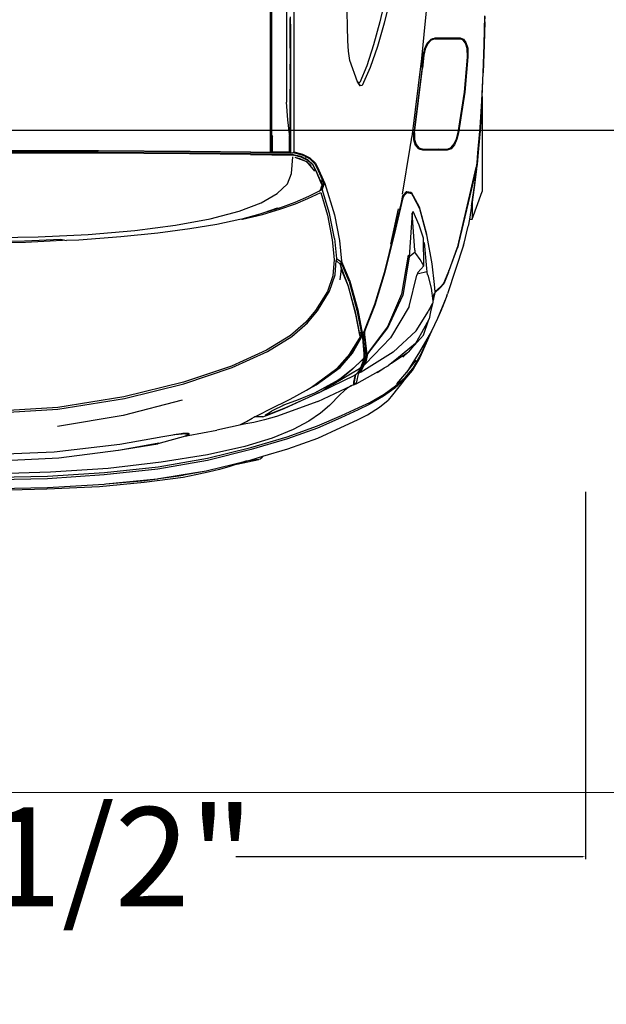
# Model space of a CAD drawing. Units: inches. Extents: x 1319 to 2030, y 219 to 1069.
# Tile 7 of 28: x 1464 to 1506, y 322 to 392. Entities that reach past the tile are written whole.
import ezdxf

# ---------------------------------------------------------------- set-up
doc = ezdxf.new("R2010")
doc.units = ezdxf.units.IN
doc.header["$MEASUREMENT"] = 0
doc.layers.get('0').update_dxf_attribs({"color": 12})
for name, color, linetype, lineweight in [('A-ANNO-DIMS', 2, 'Continuous', 18), ('A-FLOR', 8, 'Continuous', 18), ('C-PRKG-VEHC', 8, 'Continuous', 13)]:
    doc.layers.add(name, color=color, linetype=linetype, lineweight=lineweight)
doc.layers.add('Edges', color=250, linetype='Continuous')
doc.styles.get("Standard").update_dxf_attribs({"font": 'arial.ttf'})
doc.dimstyles.get("Standard").update_dxf_attribs({"dimtxt": 7, "dimasz": 0.18, "dimexe": 0.18, "dimexo": 0.0625, "dimgap": 0.09, "dimtad": 0, "dimtih": 1, "dimtoh": 1, "dimzin": 0, "dimdsep": 46, "dimlunit": 3, "dimtxsty": 'Standard', "dimcen": 0.09, "dimadec": 0, "dimazin": 0, "dimtfac": 1, "dimtofl": 0, "dimtmove": 0, "dimatfit": 3, "dimfxl": 1, "dimtolj": 1, "dimtzin": 0, "dimarcsym": 0})

# ---------------------------------------------------------------- blocks, each defined once
blk = doc.blocks.new('Nissan Qashqai pl')
at = {"layer": 'Edges'}
for p, q in [((10.8644, 12.8135), (10.8131, 12.8149)), ((10.8237, 12.8149), (10.8142, 12.8152)), ((10.8237, 12.8149), (10.864, 12.8138)), ((10.8596, 12.8138), (10.8589, 12.8138)), ((10.8642, 12.8136), (10.8596, 12.8138)), ((10.864, 12.8138), (10.8642, 12.8138)), ((10.8642, 12.8138), (10.9152, 12.812)), ((10.9158, 12.8118), (10.8644, 12.8135)), ((10.9577, 12.8101), (10.9152, 12.812)), ((10.9657, 12.8095), (10.9158, 12.8118)), ((10.9577, 12.8101), (10.9649, 12.8097)), ((10.9577, 12.8101), (11.1283, 12.8101)), ((10.9649, 12.8097), (11.0127, 12.8067)), ((11.0138, 12.8064), (10.9657, 12.8095)), ((11.0127, 12.8067), (11.0576, 12.8026)), ((11.059, 12.8023), (11.0138, 12.8064)), ((11.1783, 12.7921), (11.1283, 12.8101)), ((11.0576, 12.8026), (11.0798, 12.8008)), ((11.0768, 12.8008), (11.059, 12.8023)), ((11.0811, 12.8004), (11.0768, 12.8008)), ((11.0798, 12.8008), (11.0872, 12.7999)), ((11.0827, 12.8001), (11.0811, 12.8004)), ((11.0827, 12.8001), (11.0813, 12.7998)), ((11.0836, 12.8002), (11.0827, 12.8001)), ((11.0856, 12.7994), (11.0827, 12.8001)), ((11.0872, 12.7999), (11.0836, 12.8002)), ((11.0836, 12.8002), (11.0882, 12.7992)), ((11.2196, 12.7681), (11.0856, 12.7994)), ((11.0883, 12.7998), (11.0872, 12.7999)), ((11.0882, 12.7992), (11.2222, 12.7676)), ((11.0883, 12.7998), (11.1123, 12.797)), ((11.1147, 12.7965), (11.0883, 12.7998)), ((11.1123, 12.797), (11.1475, 12.7921)), ((11.1547, 12.791), (11.1147, 12.7965)), ((11.1475, 12.7921), (11.1525, 12.7914)), ((11.1475, 12.7921), (11.1783, 12.7921)), ((11.1525, 12.7914), (11.1547, 12.791)), ((11.1547, 12.791), (11.1783, 12.787)), ((11.1783, 12.787), (11.1783, 12.7921)), ((10.8523, 12.7704), (10.8546, 12.7762)), ((10.8523, 12.7255), (10.8523, 12.7704)), ((10.8543, 12.7702), (10.8538, 12.753)), ((10.8565, 12.7757), (10.8543, 12.7702)), ((10.8543, 12.7255), (10.8543, 12.7702)), ((10.8546, 12.7762), (10.8607, 12.7808)), ((10.8622, 12.7801), (10.8565, 12.7757)), ((10.8607, 12.7808), (10.8708, 12.7841)), ((10.8716, 12.7832), (10.8622, 12.7801)), ((10.8708, 12.7841), (10.8869, 12.7844)), ((10.887, 12.7835), (10.8716, 12.7832)), ((10.8869, 12.7844), (10.9499, 12.7789)), ((10.9498, 12.7781), (10.887, 12.7835)), ((11.0226, 12.7668), (10.9498, 12.7781)), ((10.9499, 12.7789), (11.0229, 12.7676)), ((11.1783, 12.787), (11.1906, 12.7849)), ((11.1906, 12.7849), (11.1909, 12.7849)), ((11.193, 12.7845), (11.1909, 12.7849)), ((11.2215, 12.7775), (11.193, 12.7845)), ((11.2247, 12.7764), (11.2215, 12.7775)), ((11.2247, 12.7764), (11.3124, 12.7479)), ((10.8528, 12.7503), (10.8535, 12.7521)), ((10.8535, 12.7521), (10.8538, 12.753)), ((10.8538, 12.7521), (10.8535, 12.7521)), ((10.8538, 12.753), (10.8538, 12.7521)), ((10.8538, 12.7521), (10.8538, 12.7502)), ((11.0339, 12.7639), (11.0226, 12.7668)), ((11.0229, 12.7676), (11.0348, 12.7645)), ((11.0429, 12.7597), (11.0339, 12.7639)), ((11.0348, 12.7645), (11.0444, 12.7601)), ((11.0497, 12.7542), (11.0429, 12.7597)), ((11.0444, 12.7601), (11.0516, 12.7542)), ((11.0523, 12.7475), (11.0497, 12.7542)), ((11.0516, 12.7542), (11.0543, 12.7473)), ((11.2247, 12.767), (11.2163, 12.7689)), ((11.22, 12.768), (11.2196, 12.7681)), ((11.2247, 12.767), (11.22, 12.768)), ((11.2222, 12.7676), (11.2271, 12.7664)), ((11.2253, 12.7668), (11.2247, 12.767)), ((11.2304, 12.7649), (11.2253, 12.7668)), ((11.2253, 12.7668), (11.2271, 12.7664)), ((11.2271, 12.7664), (11.2296, 12.7658)), ((11.2271, 12.7664), (11.2277, 12.7662)), ((11.2277, 12.7662), (11.2296, 12.7658)), ((11.2732, 12.7496), (11.2277, 12.7662)), ((11.2704, 12.7504), (11.2304, 12.7649)), ((10.8528, 12.742), (10.8528, 12.7503)), ((10.8528, 12.742), (10.8538, 12.742)), ((10.8528, 12.7419), (10.8528, 12.742)), ((10.8538, 12.7419), (10.8528, 12.7419)), ((10.8528, 12.7242), (10.8528, 12.7419)), ((10.8538, 12.7502), (10.8538, 12.742)), ((10.8538, 12.742), (10.8538, 12.7419)), ((10.8538, 12.7214), (10.8538, 12.7419)), ((11.0528, 12.73), (11.0523, 12.7475)), ((11.0523, 12.7312), (11.0523, 12.7475)), ((11.0543, 12.7473), (11.0543, 12.7035)), ((11.2702, 12.7507), (11.2704, 12.7504)), ((11.2704, 12.7506), (11.2707, 12.7503)), ((11.2707, 12.7503), (11.2704, 12.7504)), ((11.2719, 12.7498), (11.2707, 12.7503)), ((11.2934, 12.741), (11.2719, 12.7498)), ((11.2732, 12.7496), (11.2946, 12.7409)), ((11.3, 12.735), (11.2934, 12.741)), ((11.2946, 12.7409), (11.3018, 12.7346)), ((11.3081, 12.7253), (11.3, 12.735)), ((11.3018, 12.7346), (11.3103, 12.7249)), ((11.3161, 12.7467), (11.3124, 12.7479)), ((11.3161, 12.7467), (11.3376, 12.7381)), ((11.3192, 12.7454), (11.3566, 12.7294)), ((11.3405, 12.7369), (11.3376, 12.7381)), ((11.3405, 12.7369), (11.3566, 12.7294)), ((10.8528, 12.7242), (10.8523, 12.7255)), ((10.8538, 12.7214), (10.8528, 12.7242)), ((10.855, 12.7181), (10.8538, 12.7214)), ((10.8543, 12.7255), (10.8569, 12.7184)), ((10.8622, 12.7114), (10.855, 12.7181)), ((10.8569, 12.7184), (10.8637, 12.712)), ((11.0523, 12.7312), (11.0528, 12.73)), ((11.0523, 12.7287), (11.0523, 12.7312)), ((11.0528, 12.7274), (11.0523, 12.7287)), ((11.0523, 12.7037), (11.0523, 12.7287)), ((11.0528, 12.7274), (11.0528, 12.73)), ((11.0528, 12.73), (11.0538, 12.7273)), ((11.0528, 12.7274), (11.0528, 12.6985)), ((11.0538, 12.7273), (11.0538, 12.7018)), ((11.2091, 12.7103), (11.2583, 12.7196)), ((11.2583, 12.7196), (11.2956, 12.7234)), ((11.2787, 12.7123), (11.3022, 12.7186)), ((11.2956, 12.7234), (11.3085, 12.7247)), ((11.3022, 12.7186), (11.3252, 12.7213)), ((11.3086, 12.7247), (11.3081, 12.7253)), ((11.3081, 12.7253), (11.3087, 12.7247)), ((11.3085, 12.7247), (11.3086, 12.7247)), ((11.3086, 12.7247), (11.3087, 12.7247)), ((11.3087, 12.7247), (11.3103, 12.7249)), ((11.3103, 12.7249), (11.3103, 12.7249)), ((11.3103, 12.7249), (11.3106, 12.7249)), ((11.3106, 12.7249), (11.314, 12.7238)), ((11.317, 12.7227), (11.3119, 12.7236)), ((11.3132, 12.7243), (11.3256, 12.7215)), ((11.314, 12.7238), (11.317, 12.7227)), ((11.314, 12.7238), (11.3242, 12.7216)), ((11.3242, 12.7216), (11.317, 12.7227)), ((11.3198, 12.7211), (11.3252, 12.7213)), ((11.3242, 12.7216), (11.3256, 12.7215)), ((11.3252, 12.7213), (11.3283, 12.7214)), ((11.3256, 12.7215), (11.3283, 12.7214)), ((11.3283, 12.7214), (11.3297, 12.7206)), ((11.3297, 12.7206), (11.3446, 12.7173)), ((11.3297, 12.7206), (11.3302, 12.7203)), ((11.3302, 12.7203), (11.3446, 12.7173)), ((11.3302, 12.7203), (11.3394, 12.7152)), ((11.3446, 12.7173), (11.3571, 12.7146)), ((11.3566, 12.7294), (11.3796, 12.7187)), ((11.3796, 12.7187), (11.4164, 12.6974)), ((11.3796, 12.7187), (11.3807, 12.7182)), ((11.3807, 12.7182), (11.4267, 12.6979)), ((11.4228, 12.6989), (11.3807, 12.7182)), ((10.7615, 12.7131), (10.8218, 12.7077)), ((10.8218, 12.7077), (10.8896, 12.7008)), ((10.8718, 12.7068), (10.8622, 12.7114)), ((10.8637, 12.712), (10.8727, 12.7077)), ((10.8836, 12.7041), (10.8718, 12.7068)), ((10.8727, 12.7077), (10.8839, 12.7051)), ((10.9054, 12.702), (10.8836, 12.7041)), ((10.8839, 12.7051), (10.9067, 12.7029)), ((10.8896, 12.7008), (11.0304, 12.6838)), ((10.9054, 12.702), (11.0232, 12.6871)), ((11.0231, 12.6882), (10.9067, 12.7029)), ((11.0501, 12.6964), (11.0523, 12.7037)), ((11.0538, 12.7018), (11.0528, 12.6985)), ((11.0543, 12.7035), (11.0538, 12.7018)), ((11.156, 12.6966), (11.203, 12.7093)), ((11.1589, 12.6971), (11.2062, 12.7098)), ((11.2121, 12.7043), (11.189, 12.6968)), ((11.203, 12.7093), (11.2091, 12.7103)), ((11.2062, 12.7098), (11.2091, 12.7103)), ((11.2622, 12.7051), (11.2121, 12.7043)), ((11.2199, 12.706), (11.2666, 12.7097)), ((11.2601, 12.7037), (11.2505, 12.6987)), ((11.2622, 12.7051), (11.2601, 12.7037)), ((11.2743, 12.6942), (11.2622, 12.7051)), ((11.2666, 12.7097), (11.2729, 12.7104)), ((11.2787, 12.7123), (11.2729, 12.7104)), ((11.2729, 12.7104), (11.2766, 12.6957)), ((11.3394, 12.7152), (11.3434, 12.7138)), ((11.3394, 12.7152), (11.342, 12.7137)), ((11.379, 12.6915), (11.3434, 12.7138)), ((11.3583, 12.7142), (11.3571, 12.7146)), ((11.3571, 12.7146), (11.3821, 12.7008)), ((11.3583, 12.7142), (11.3821, 12.7008)), ((11.3864, 12.7044), (11.3583, 12.7142)), ((11.3821, 12.7008), (11.4014, 12.69)), ((11.4163, 12.6775), (11.3864, 12.7044)), ((11.0231, 12.6882), (11.035, 12.6883)), ((11.0358, 12.6872), (11.0232, 12.6871)), ((11.0357, 12.6829), (11.0304, 12.6838)), ((11.035, 12.6883), (11.0443, 12.6911)), ((11.0491, 12.6807), (11.0357, 12.6829)), ((11.0458, 12.6903), (11.0358, 12.6872)), ((11.0443, 12.6911), (11.0501, 12.6964)), ((11.052, 12.6958), (11.0458, 12.6903)), ((11.0528, 12.6985), (11.052, 12.6958)), ((11.1285, 12.6745), (11.1298, 12.6823)), ((11.1298, 12.6823), (11.156, 12.6966)), ((11.1306, 12.6752), (11.1319, 12.6827)), ((11.1319, 12.6827), (11.1306, 12.6812)), ((11.1319, 12.6827), (11.1365, 12.6851)), ((11.1365, 12.6851), (11.1589, 12.6971)), ((11.189, 12.6968), (11.1644, 12.6862)), ((11.1644, 12.6862), (11.1672, 12.6844)), ((11.2337, 12.6892), (11.1672, 12.6844)), ((11.1672, 12.6844), (11.2459, 12.6785)), ((11.2337, 12.6892), (11.2382, 12.6892)), ((11.2382, 12.6892), (11.2401, 12.6908)), ((11.2382, 12.6892), (11.2459, 12.6785)), ((11.2505, 12.6987), (11.2401, 12.6908)), ((11.2743, 12.6942), (11.2791, 12.6927)), ((11.335, 12.6786), (11.2791, 12.6927)), ((11.379, 12.6915), (11.417, 12.6499)), ((11.4014, 12.69), (11.4022, 12.6894)), ((11.4014, 12.69), (11.4265, 12.6594)), ((11.4022, 12.6894), (11.4163, 12.6775)), ((11.4022, 12.6894), (11.4265, 12.6594)), ((11.4164, 12.6974), (11.4531, 12.6744)), ((11.4243, 12.6982), (11.4228, 12.6989)), ((11.4464, 12.6853), (11.4243, 12.6982)), ((11.4267, 12.6979), (11.4498, 12.6844)), ((11.4531, 12.6744), (11.4314, 12.6911)), ((11.4624, 12.6717), (11.4464, 12.6853)), ((11.4498, 12.6844), (11.4662, 12.6706)), ((11.4681, 12.6691), (11.4498, 12.6844)), ((11.0449, 12.6812), (11.0448, 12.6812)), ((11.0492, 12.6807), (11.0491, 12.6807)), ((11.1336, 12.667), (11.0492, 12.6807)), ((11.1293, 12.6736), (11.1285, 12.6745)), ((11.1306, 12.6812), (11.1293, 12.6736)), ((11.1353, 12.6677), (11.1293, 12.6736)), ((11.1347, 12.671), (11.1306, 12.6752)), ((11.1366, 12.6691), (11.1347, 12.671)), ((11.1358, 12.6676), (11.1353, 12.6677)), ((11.1358, 12.6676), (11.1366, 12.6691)), ((11.148, 12.665), (11.1358, 12.6676)), ((11.1401, 12.6682), (11.1366, 12.6691)), ((11.2066, 12.6527), (11.1401, 12.6682)), ((11.2063, 12.6515), (11.148, 12.665)), ((11.2428, 12.6769), (11.3132, 12.6652)), ((11.2459, 12.6785), (11.3153, 12.6672)), ((11.3132, 12.6652), (11.3715, 12.6398)), ((11.3733, 12.6404), (11.3153, 12.6672)), ((11.335, 12.6786), (11.3915, 12.6453)), ((11.4366, 12.6471), (11.4163, 12.6775)), ((11.4163, 12.6775), (11.4259, 12.6674)), ((11.4742, 12.6567), (11.4531, 12.6744)), ((11.4774, 12.6543), (11.4624, 12.6717)), ((11.4662, 12.6706), (11.4815, 12.6531)), ((11.4681, 12.6691), (11.4936, 12.6491)), ((10.7776, 12.646), (10.8264, 12.6341)), ((11.2232, 12.6458), (11.1598, 12.6594)), ((11.272, 12.6349), (11.2063, 12.6515)), ((11.2728, 12.6357), (11.2066, 12.6527)), ((11.417, 12.6499), (11.4529, 12.5922)), ((11.4265, 12.6594), (11.4366, 12.6471)), ((11.4366, 12.6471), (11.4408, 12.6419)), ((11.4924, 12.6339), (11.4774, 12.6543)), ((11.4815, 12.6531), (11.4963, 12.6328)), ((11.4936, 12.6491), (11.5033, 12.6408)), ((10.7754, 12.637), (10.8239, 12.6261)), ((10.8264, 12.6341), (10.8682, 12.6216)), ((11.3311, 12.6172), (11.272, 12.6349)), ((11.3323, 12.6178), (11.2728, 12.6357)), ((11.3715, 12.6398), (11.4177, 12.6052)), ((11.4203, 12.6044), (11.3733, 12.6404)), ((11.3915, 12.6453), (11.4381, 12.6002)), ((11.4408, 12.6419), (11.4411, 12.6414)), ((11.4411, 12.6414), (11.4411, 12.6414)), ((11.4414, 12.6409), (11.4411, 12.6414)), ((11.4414, 12.6409), (11.447, 12.6315)), ((11.4455, 12.6336), (11.4414, 12.6409)), ((11.447, 12.6315), (11.4455, 12.6336)), ((11.4455, 12.6336), (11.4462, 12.6324)), ((11.447, 12.6315), (11.4462, 12.6324)), ((11.4732, 12.585), (11.4462, 12.6324)), ((11.447, 12.6315), (11.447, 12.6314)), ((11.4536, 12.6215), (11.447, 12.6314)), ((11.5074, 12.608), (11.4924, 12.6339)), ((11.4964, 12.6326), (11.4963, 12.6328)), ((11.4964, 12.6326), (11.5113, 12.6069)), ((11.5158, 12.6256), (11.5033, 12.6408)), ((10.8239, 12.6261), (10.8653, 12.6144)), ((10.8653, 12.6144), (10.9026, 12.6025)), ((10.8682, 12.6216), (10.9059, 12.6087)), ((11.3751, 12.5999), (11.3311, 12.6172)), ((11.3747, 12.6011), (11.3323, 12.6178)), ((11.5295, 12.6041), (11.5158, 12.6256)), ((10.9026, 12.6025), (10.933, 12.5901)), ((10.9059, 12.6087), (10.9384, 12.5945)), ((10.9384, 12.5945), (10.9386, 12.5905)), ((11.3411, 12.5863), (11.3795, 12.5939)), ((11.38, 12.5988), (11.3747, 12.6011)), ((11.3751, 12.5999), (11.3762, 12.5999)), ((11.3752, 12.5998), (11.3751, 12.5999)), ((11.3763, 12.5998), (11.3752, 12.5998)), ((11.3764, 12.5993), (11.3752, 12.5998)), ((11.3792, 12.5982), (11.3764, 12.5993)), ((11.3792, 12.5982), (11.3793, 12.5979)), ((11.3792, 12.5982), (11.3804, 12.5972)), ((11.3795, 12.5939), (11.3834, 12.5947)), ((11.3853, 12.5993), (11.38, 12.5988)), ((11.3804, 12.5972), (11.4082, 12.5998)), ((11.3827, 12.5953), (11.3804, 12.5972)), ((11.3804, 12.5926), (11.3841, 12.5933)), ((11.3811, 12.5958), (11.3808, 12.5961)), ((11.3834, 12.5947), (11.3827, 12.5953)), ((11.3846, 12.5953), (11.3829, 12.5952)), ((11.3829, 12.5952), (11.3849, 12.5951)), ((11.388, 12.591), (11.3829, 12.5952)), ((11.3834, 12.5947), (11.3841, 12.5933)), ((11.3846, 12.5953), (11.4248, 12.5976)), ((11.3846, 12.5953), (11.3846, 12.5953)), ((11.3851, 12.5951), (11.3846, 12.5953)), ((11.3846, 12.5953), (11.3849, 12.5951)), ((11.3849, 12.5951), (11.3851, 12.5951)), ((11.3882, 12.5923), (11.3849, 12.5951)), ((11.3851, 12.5951), (11.3867, 12.5949)), ((11.4171, 12.5766), (11.3851, 12.5951)), ((11.4212, 12.603), (11.3853, 12.5993)), ((11.3867, 12.5949), (11.3915, 12.5951)), ((11.3914, 12.5926), (11.3867, 12.5949)), ((11.3915, 12.5951), (11.4266, 12.5977)), ((11.409, 12.5999), (11.4082, 12.5998)), ((11.4164, 12.5998), (11.4082, 12.5998)), ((11.4152, 12.6004), (11.409, 12.5999)), ((11.409, 12.5999), (11.4163, 12.5999)), ((11.4173, 12.6006), (11.4152, 12.6004)), ((11.4163, 12.5999), (11.4152, 12.6004)), ((11.4163, 12.5999), (11.4186, 12.5999)), ((11.4164, 12.5998), (11.4163, 12.5999)), ((11.4181, 12.5998), (11.4164, 12.5998)), ((11.4169, 12.5996), (11.4164, 12.5998)), ((11.4252, 12.598), (11.4169, 12.5996)), ((11.4176, 12.6007), (11.4173, 12.6006)), ((11.418, 12.6006), (11.4173, 12.6006)), ((11.4215, 12.601), (11.4176, 12.6007)), ((11.418, 12.6006), (11.4176, 12.6007)), ((11.4177, 12.6052), (11.4193, 12.6042)), ((11.4204, 12.6002), (11.418, 12.6006)), ((11.4194, 12.6), (11.418, 12.6006)), ((11.4192, 12.6045), (11.4194, 12.6042)), ((11.4194, 12.6042), (11.4193, 12.6042)), ((11.4193, 12.6042), (11.4196, 12.604)), ((11.4194, 12.6042), (11.4196, 12.604)), ((11.4196, 12.6042), (11.4194, 12.6042)), ((11.4196, 12.604), (11.4201, 12.6036)), ((11.4198, 12.6041), (11.4201, 12.6036)), ((11.4201, 12.6036), (11.4212, 12.603)), ((11.4292, 12.6024), (11.4203, 12.6044)), ((11.4229, 12.6025), (11.4203, 12.6044)), ((11.4212, 12.603), (11.4215, 12.601)), ((11.4218, 12.6028), (11.4212, 12.603)), ((11.4215, 12.601), (11.4219, 12.6009)), ((11.4222, 12.6029), (11.4218, 12.6028)), ((11.4229, 12.6025), (11.4218, 12.6028)), ((11.4219, 12.6009), (11.4222, 12.6005)), ((11.4219, 12.6009), (11.4224, 12.6008)), ((11.4224, 12.6008), (11.4226, 12.6006)), ((11.4224, 12.6008), (11.423, 12.6006)), ((11.4315, 12.6002), (11.4229, 12.6025)), ((11.423, 12.6006), (11.4229, 12.6025)), ((11.44, 12.5959), (11.423, 12.6006)), ((11.4248, 12.5976), (11.4266, 12.5977)), ((11.4266, 12.5977), (11.4252, 12.598)), ((11.4266, 12.5977), (11.4268, 12.5977)), ((11.4268, 12.5977), (11.4296, 12.5954)), ((11.4268, 12.5977), (11.4278, 12.5977)), ((11.4303, 12.5956), (11.4278, 12.5977)), ((11.4278, 12.5977), (11.43, 12.5969)), ((11.4381, 12.6002), (11.4292, 12.6024)), ((11.4296, 12.5954), (11.4469, 12.5773)), ((11.4337, 12.5962), (11.43, 12.5969)), ((11.43, 12.5969), (11.4361, 12.5948)), ((11.4479, 12.5766), (11.4303, 12.5956)), ((11.4403, 12.5978), (11.4315, 12.6002)), ((11.4397, 12.5937), (11.4337, 12.5962)), ((11.4361, 12.5948), (11.4406, 12.5932)), ((11.4381, 12.6002), (11.4403, 12.5978)), ((11.4406, 12.5932), (11.4397, 12.5937)), ((11.4403, 12.5978), (11.44, 12.5959)), ((11.44, 12.5959), (11.4457, 12.5928)), ((11.4462, 12.5947), (11.4403, 12.5978)), ((11.4406, 12.5932), (11.4442, 12.592)), ((11.4457, 12.5928), (11.4512, 12.5893)), ((11.452, 12.591), (11.4462, 12.5947)), ((11.5165, 12.5882), (11.5074, 12.608)), ((11.5113, 12.6068), (11.5113, 12.6069)), ((11.5113, 12.6068), (11.5206, 12.5869)), ((11.5384, 12.5859), (11.5295, 12.6041)), ((10.9316, 12.586), (10.8932, 12.572)), ((10.9316, 12.586), (10.9334, 12.5872)), ((10.932, 12.5862), (10.9316, 12.586)), ((10.9335, 12.5871), (10.932, 12.5862)), ((10.933, 12.5901), (10.9334, 12.5872)), ((10.9334, 12.5872), (10.9386, 12.5905)), ((10.9334, 12.5872), (10.9335, 12.5871)), ((10.9386, 12.5905), (10.9335, 12.5871)), ((11.2895, 12.5724), (11.3411, 12.5863)), ((11.29, 12.5711), (11.3419, 12.585)), ((11.3474, 12.5827), (11.2972, 12.5692)), ((11.3493, 12.5828), (11.2993, 12.5695)), ((11.3419, 12.585), (11.3804, 12.5926)), ((11.3847, 12.5899), (11.3474, 12.5827)), ((11.3474, 12.5827), (11.3474, 12.5827)), ((11.3863, 12.5898), (11.3493, 12.5828)), ((11.3847, 12.5899), (11.3804, 12.5926)), ((11.3847, 12.5899), (11.3848, 12.5899)), ((11.388, 12.591), (11.3848, 12.5899)), ((11.3895, 12.5912), (11.3863, 12.5898)), ((11.3886, 12.5919), (11.3872, 12.5927)), ((11.3882, 12.5923), (11.3886, 12.5919)), ((11.3886, 12.5919), (11.3895, 12.5912)), ((11.3892, 12.5916), (11.3886, 12.5919)), ((11.3923, 12.5894), (11.3895, 12.5912)), ((11.4187, 12.5768), (11.3914, 12.5926)), ((11.4203, 12.5724), (11.3923, 12.5894)), ((11.4433, 12.5543), (11.4171, 12.5766)), ((11.4447, 12.5545), (11.4187, 12.5768)), ((11.4442, 12.592), (11.4497, 12.589)), ((11.4462, 12.5893), (11.4442, 12.592)), ((11.475, 12.5409), (11.4462, 12.5893)), ((11.4469, 12.5773), (11.4659, 12.5539)), ((11.4654, 12.5548), (11.4479, 12.5766)), ((11.4497, 12.589), (11.4498, 12.5889)), ((11.4535, 12.5876), (11.4498, 12.5889)), ((11.4498, 12.5889), (11.4549, 12.5855)), ((11.4512, 12.5893), (11.4535, 12.5876)), ((11.4539, 12.5897), (11.452, 12.591)), ((11.4529, 12.5922), (11.4542, 12.5894)), ((11.4535, 12.5876), (11.4532, 12.5882)), ((11.4535, 12.5876), (11.4542, 12.5894)), ((11.4535, 12.5876), (11.4728, 12.5838)), ((11.4542, 12.5894), (11.4539, 12.5897)), ((11.4549, 12.5855), (11.4568, 12.5836)), ((11.4564, 12.5833), (11.4567, 12.5833)), ((11.4569, 12.583), (11.4565, 12.5831)), ((11.4568, 12.5836), (11.4571, 12.5833)), ((11.4571, 12.5833), (11.4573, 12.583)), ((11.4573, 12.583), (11.4578, 12.5822)), ((11.4704, 12.5803), (11.4573, 12.583)), ((11.4573, 12.5823), (11.4574, 12.5822)), ((11.4573, 12.5823), (11.4573, 12.5823)), ((11.4576, 12.5822), (11.4574, 12.5822)), ((11.4578, 12.5822), (11.4588, 12.5807)), ((11.4605, 12.5816), (11.4578, 12.5822)), ((11.4588, 12.5807), (11.4895, 12.5178)), ((11.4713, 12.5794), (11.4605, 12.5816)), ((11.4742, 12.5797), (11.4704, 12.5803)), ((11.4744, 12.5792), (11.4713, 12.5794)), ((11.4732, 12.585), (11.4728, 12.5838)), ((11.4728, 12.5838), (11.4742, 12.5797)), ((11.4728, 12.5838), (11.4746, 12.5796)), ((11.4758, 12.5791), (11.4732, 12.585)), ((11.4742, 12.5797), (11.4744, 12.5792)), ((11.4745, 12.5797), (11.4742, 12.5797)), ((11.4745, 12.5792), (11.4744, 12.5792)), ((11.4745, 12.5792), (11.4745, 12.5797)), ((11.4745, 12.5797), (11.4746, 12.5796)), ((11.4748, 12.5792), (11.4745, 12.5792)), ((11.4746, 12.5796), (11.4748, 12.5792)), ((11.4746, 12.5796), (11.4758, 12.5791)), ((11.4758, 12.5791), (11.4748, 12.5792)), ((11.4758, 12.5791), (11.4759, 12.579)), ((11.4759, 12.579), (11.4778, 12.5746)), ((11.4759, 12.579), (11.4771, 12.576)), ((11.5057, 12.5145), (11.4771, 12.576)), ((11.5306, 12.5573), (11.5165, 12.5882)), ((11.5206, 12.5869), (11.5349, 12.5559)), ((11.5527, 12.5559), (11.5384, 12.5859)), ((10.858, 12.5683), (10.7769, 12.5667)), ((10.8766, 12.5697), (10.858, 12.5683)), ((10.8932, 12.572), (10.8766, 12.5697)), ((11.2538, 12.5571), (11.2586, 12.5591)), ((11.29, 12.5711), (11.2541, 12.5557)), ((11.2586, 12.5591), (11.2895, 12.5724)), ((11.2705, 12.5579), (11.265, 12.5563)), ((11.2972, 12.5692), (11.2677, 12.5575)), ((11.2993, 12.5695), (11.2705, 12.5579)), ((11.4467, 12.5488), (11.4203, 12.5724)), ((11.4633, 12.5594), (11.4897, 12.5108)), ((11.4778, 12.5746), (11.4826, 12.5669)), ((11.4826, 12.5669), (11.4869, 12.5615)), ((11.4869, 12.5615), (11.4933, 12.555)), ((11.1144, 12.5271), (11.1702, 12.5444)), ((11.2127, 12.5443), (11.1683, 12.5354)), ((11.1702, 12.5444), (11.2166, 12.5534)), ((11.1712, 12.5317), (11.2152, 12.5404)), ((11.2127, 12.5443), (11.2488, 12.548)), ((11.2152, 12.5404), (11.2509, 12.5439)), ((11.2166, 12.5534), (11.2538, 12.5571)), ((11.2488, 12.548), (11.2541, 12.5557)), ((11.2488, 12.548), (11.2524, 12.5477)), ((11.2509, 12.5439), (11.28, 12.5414)), ((11.2599, 12.5552), (11.2524, 12.5477)), ((11.2785, 12.5455), (11.2524, 12.5477)), ((11.2541, 12.5557), (11.2599, 12.5552)), ((11.2677, 12.5575), (11.2599, 12.5552)), ((11.265, 12.5563), (11.2599, 12.5552)), ((11.265, 12.5563), (11.2724, 12.5557)), ((11.2724, 12.5557), (11.2874, 12.5544)), ((11.3076, 12.5358), (11.2785, 12.5455)), ((11.28, 12.5414), (11.3082, 12.532)), ((11.4745, 12.5116), (11.4433, 12.5543)), ((11.4758, 12.5118), (11.4447, 12.5545)), ((11.4801, 12.503), (11.4467, 12.5488)), ((11.4654, 12.5548), (11.4659, 12.5539)), ((11.4659, 12.5539), (11.4674, 12.5512)), ((11.4675, 12.551), (11.4674, 12.5512)), ((11.4675, 12.551), (11.4703, 12.546)), ((11.4703, 12.546), (11.4704, 12.5458)), ((11.4704, 12.5458), (11.4909, 12.5085)), ((11.4704, 12.5458), (11.4897, 12.5108)), ((11.475, 12.5409), (11.4828, 12.5276)), ((11.5131, 12.5356), (11.4933, 12.555)), ((11.5496, 12.5141), (11.5306, 12.5573)), ((11.5349, 12.5559), (11.5535, 12.5139)), ((11.5716, 12.5145), (11.5527, 12.5559)), ((11.0902, 12.5166), (11.1144, 12.5271)), ((11.0908, 12.5153), (11.107, 12.5224)), ((11.107, 12.5224), (11.1116, 12.5243)), ((11.1138, 12.5213), (11.107, 12.5224)), ((11.1116, 12.5243), (11.1147, 12.5257)), ((11.1244, 12.5227), (11.1116, 12.5243)), ((11.1164, 12.5224), (11.1139, 12.5213)), ((11.1147, 12.5257), (11.1244, 12.5227)), ((11.1172, 12.5222), (11.1149, 12.5212)), ((11.1164, 12.5224), (11.1174, 12.5223)), ((11.1173, 12.5222), (11.1172, 12.5222)), ((11.1174, 12.5223), (11.1173, 12.5222)), ((11.12, 12.5215), (11.1174, 12.5223)), ((11.1683, 12.5354), (11.1244, 12.5227)), ((11.1259, 12.5194), (11.1244, 12.5227)), ((11.1244, 12.5227), (11.126, 12.5194)), ((11.1302, 12.52), (11.1712, 12.5317)), ((11.3428, 12.5139), (11.3076, 12.5358)), ((11.3082, 12.532), (11.3425, 12.5106)), ((11.488, 12.5208), (11.4828, 12.5276)), ((11.5131, 12.5356), (11.5265, 12.5194)), ((11.0682, 12.5004), (11.0779, 12.5103)), ((11.0692, 12.4996), (11.0787, 12.5092)), ((11.0802, 12.5057), (11.0718, 12.4967)), ((11.0809, 12.5056), (11.0727, 12.4966)), ((11.0747, 12.4944), (11.092, 12.5087)), ((11.0779, 12.5103), (11.0902, 12.5166)), ((11.0787, 12.5092), (11.0908, 12.5153)), ((11.0912, 12.5117), (11.0802, 12.5057)), ((11.0917, 12.5114), (11.0809, 12.5056)), ((11.1138, 12.5213), (11.0912, 12.5117)), ((11.1149, 12.5212), (11.0917, 12.5114)), ((11.1139, 12.5213), (11.1138, 12.5213)), ((11.1246, 12.5199), (11.12, 12.5215)), ((11.1259, 12.5194), (11.1246, 12.5199)), ((11.126, 12.5193), (11.1247, 12.5197)), ((11.126, 12.5193), (11.1248, 12.5195)), ((11.1251, 12.5189), (11.126, 12.5193)), ((11.126, 12.5193), (11.1259, 12.5194)), ((11.126, 12.5194), (11.1259, 12.5194)), ((11.126, 12.5194), (11.1261, 12.5193)), ((11.1264, 12.5192), (11.126, 12.5194)), ((11.1263, 12.5186), (11.126, 12.5193)), ((11.1261, 12.5193), (11.126, 12.5193)), ((11.1261, 12.5193), (11.1263, 12.5188)), ((11.1264, 12.5192), (11.1261, 12.5193)), ((11.1277, 12.5167), (11.1264, 12.5192)), ((11.1369, 12.4986), (11.1277, 12.5167)), ((11.1412, 12.4969), (11.1302, 12.52)), ((11.3425, 12.5106), (11.3635, 12.4929)), ((11.3645, 12.4958), (11.3428, 12.5139)), ((11.4788, 12.5052), (11.4745, 12.5116)), ((11.4852, 12.494), (11.4758, 12.5118)), ((11.4801, 12.503), (11.4788, 12.5052)), ((11.5179, 12.4551), (11.488, 12.5208)), ((11.4898, 12.5172), (11.4895, 12.5178)), ((11.4897, 12.5108), (11.4909, 12.5085)), ((11.4898, 12.5172), (11.49, 12.5167)), ((11.49, 12.5167), (11.5179, 12.4551)), ((11.4909, 12.5085), (11.5028, 12.4792)), ((11.5057, 12.5145), (11.5325, 12.4404)), ((11.5265, 12.5194), (11.541, 12.4982)), ((11.5691, 12.4592), (11.5496, 12.5141)), ((11.5535, 12.5139), (11.5726, 12.46)), ((11.5908, 12.4606), (11.5716, 12.5145)), ((11.0581, 12.4738), (11.0614, 12.4872)), ((11.0614, 12.4872), (11.0682, 12.5004)), ((11.0624, 12.4866), (11.0658, 12.4932)), ((11.0658, 12.4932), (11.0692, 12.4996)), ((11.0658, 12.4932), (11.0698, 12.4925)), ((11.0698, 12.4925), (11.0659, 12.4848)), ((11.0727, 12.4966), (11.0669, 12.4849)), ((11.0671, 12.4731), (11.0747, 12.4944)), ((11.0696, 12.4836), (11.0747, 12.4944)), ((11.0718, 12.4967), (11.0698, 12.4925)), ((11.0747, 12.4944), (11.0821, 12.5029)), ((11.1475, 12.4741), (11.1369, 12.4986)), ((11.1505, 12.4742), (11.1412, 12.4969)), ((11.3635, 12.4929), (11.3872, 12.4654)), ((11.3888, 12.4678), (11.3645, 12.4958)), ((11.4852, 12.494), (11.4801, 12.503)), ((11.5013, 12.4651), (11.4852, 12.494)), ((11.541, 12.4982), (11.5562, 12.4701)), ((10.7004, 12.4722), (10.8279, 12.4715)), ((10.8279, 12.4715), (11.0544, 12.4714)), ((11.0544, 12.4714), (11.0575, 12.4714)), ((11.0575, 12.4714), (11.0581, 12.4738)), ((11.0575, 12.4714), (11.0582, 12.47)), ((11.0582, 12.47), (11.0624, 12.4866)), ((11.0592, 12.4653), (11.0582, 12.47)), ((11.0618, 12.3933), (11.0632, 12.47)), ((11.0622, 12.4697), (11.0621, 12.4657)), ((11.063, 12.4728), (11.0622, 12.4697)), ((11.0659, 12.4848), (11.063, 12.4728)), ((11.0641, 12.4733), (11.0632, 12.47)), ((11.0669, 12.4849), (11.0641, 12.4733)), ((11.0962, 12.4675), (11.0662, 12.4698)), ((11.0671, 12.4731), (11.0696, 12.4836)), ((11.1577, 12.4465), (11.1475, 12.4741)), ((11.1605, 12.4465), (11.1505, 12.4742)), ((11.5028, 12.4792), (11.5118, 12.4548)), ((11.5562, 12.4701), (11.5715, 12.4326)), ((10.7502, 12.4586), (10.968, 12.4585)), ((10.8279, 12.4654), (10.8145, 12.4655)), ((10.8277, 12.4647), (10.8179, 12.4648)), ((10.8711, 12.4646), (10.8277, 12.4647)), ((10.8279, 12.4654), (11.0592, 12.4653)), ((10.8711, 12.4646), (10.8824, 12.4646)), ((10.8824, 12.4646), (10.8825, 12.4646)), ((10.8825, 12.4646), (10.8884, 12.4646)), ((10.8884, 12.4646), (10.8923, 12.4646)), ((10.8923, 12.4646), (10.8996, 12.4646)), ((10.9097, 12.4646), (10.8996, 12.4646)), ((10.9097, 12.4646), (10.9399, 12.4646)), ((10.9399, 12.4646), (10.9491, 12.4645)), ((10.9491, 12.4645), (11.0301, 12.4645)), ((11, 12.4605), (10.968, 12.4585)), ((11.0301, 12.4645), (11, 12.4605)), ((11.0301, 12.4637), (11.0287, 12.4637)), ((11.03, 12.4635), (11.0301, 12.4637)), ((11.0301, 12.4642), (11.0301, 12.4645)), ((11.0574, 12.4637), (11.0301, 12.4637)), ((11.0568, 12.4323), (11.0574, 12.4637)), ((11.0574, 12.4637), (11.0592, 12.4653)), ((11.0585, 12.43), (11.0592, 12.4653)), ((11.0621, 12.4657), (11.0607, 12.3933)), ((11.1148, 12.4598), (11.0962, 12.4675)), ((11.1323, 12.4415), (11.1148, 12.4598)), ((11.3872, 12.4654), (11.4138, 12.4223)), ((11.4159, 12.4242), (11.3888, 12.4678)), ((11.5202, 12.427), (11.5013, 12.4651)), ((11.5118, 12.4548), (11.523, 12.4311)), ((11.5118, 12.4548), (11.513, 12.4514)), ((11.5292, 12.4272), (11.5179, 12.4551)), ((11.5179, 12.4551), (11.5285, 12.4279)), ((11.5884, 12.3943), (11.5691, 12.4592)), ((11.5726, 12.46), (11.5922, 12.3947)), ((11.6042, 12.4156), (11.5908, 12.4606)), ((11.0295, 12.4341), (11.0295, 12.4343)), ((11.1487, 12.4126), (11.1323, 12.4415)), ((11.1643, 12.425), (11.1576, 12.4459)), ((11.1643, 12.425), (11.1577, 12.4465)), ((11.1582, 12.4416), (11.1668, 12.4177)), ((11.1583, 12.4423), (11.1643, 12.425)), ((11.1699, 12.4153), (11.1605, 12.4465)), ((11.5325, 12.4404), (11.5386, 12.4187)), ((10.827, 12.4297), (10.6999, 12.4304)), ((10.7493, 12.4316), (11.0294, 12.4315)), ((10.7933, 12.4303), (10.8267, 12.4301)), ((10.8267, 12.4301), (11.0585, 12.43)), ((10.9133, 12.4296), (10.827, 12.4297)), ((10.9133, 12.4296), (10.9133, 12.4298)), ((10.9137, 12.4296), (10.9133, 12.4296)), ((10.9137, 12.4296), (10.9138, 12.4298)), ((10.9715, 12.4296), (10.9137, 12.4296)), ((10.9715, 12.4299), (10.9715, 12.4296)), ((11.0579, 12.4296), (10.9715, 12.4296)), ((11.0281, 12.4323), (11.0568, 12.4323)), ((11.0294, 12.4315), (11.0294, 12.4316)), ((11.0568, 12.4323), (11.0585, 12.43)), ((11.0572, 12.3942), (11.0579, 12.4296)), ((11.0579, 12.3938), (11.0585, 12.43)), ((11.0579, 12.4296), (11.0585, 12.43)), ((11.1643, 12.425), (11.1668, 12.4177)), ((11.1668, 12.4177), (11.1694, 12.4104)), ((11.4138, 12.4223), (11.4422, 12.3594)), ((11.4445, 12.3608), (11.4159, 12.4242)), ((11.5283, 12.4109), (11.5202, 12.427)), ((11.5301, 12.4198), (11.523, 12.4311)), ((11.5285, 12.4279), (11.5302, 12.4209)), ((11.5331, 12.4157), (11.5292, 12.4272)), ((11.5302, 12.4209), (11.5301, 12.4198)), ((11.5386, 12.4187), (11.5434, 12.3997)), ((11.5715, 12.4326), (11.5866, 12.3835)), ((11.164, 12.373), (11.1487, 12.4126)), ((11.1694, 12.4104), (11.1781, 12.3782)), ((11.178, 12.379), (11.1699, 12.4153)), ((11.5334, 12.4014), (11.5283, 12.4109)), ((11.5326, 12.4045), (11.5333, 12.4019)), ((11.5331, 12.4157), (11.5335, 12.401)), ((11.5333, 12.4019), (11.5334, 12.4014)), ((11.5335, 12.401), (11.5334, 12.4014)), ((11.5357, 12.3968), (11.5335, 12.401)), ((11.5434, 12.3997), (11.5461, 12.3854)), ((11.6042, 12.4156), (11.6077, 12.4125)), ((11.6103, 12.395), (11.6042, 12.4156)), ((11.6077, 12.4125), (11.6094, 12.4107)), ((11.6094, 12.4107), (11.6101, 12.4085)), ((11.6101, 12.4085), (11.6127, 12.3852)), ((11.6185, 12.3689), (11.6101, 12.4085)), ((11.056, 12.2851), (11.0572, 12.3942)), ((11.0566, 12.2849), (11.0579, 12.3938)), ((11.0607, 12.3933), (11.0595, 12.2842)), ((11.0618, 12.3933), (11.0606, 12.2841)), ((11.5416, 12.3863), (11.5357, 12.3968)), ((11.5455, 12.3793), (11.5416, 12.3863)), ((11.5461, 12.3854), (11.5467, 12.3822)), ((11.5467, 12.3822), (11.5571, 12.3331)), ((11.5866, 12.3835), (11.6016, 12.3166)), ((11.6076, 12.3166), (11.5884, 12.3943)), ((11.5922, 12.3947), (11.6118, 12.3165)), ((11.6127, 12.3852), (11.6103, 12.395)), ((11.6127, 12.3852), (11.6174, 12.3722)), ((11.6297, 12.3166), (11.6127, 12.3852)), ((11.1776, 12.3211), (11.164, 12.373)), ((11.1781, 12.3782), (11.178, 12.379)), ((11.1781, 12.3782), (11.1791, 12.3746)), ((11.1791, 12.3746), (11.1877, 12.333)), ((11.5472, 12.3757), (11.5455, 12.3793)), ((11.6174, 12.3722), (11.6185, 12.3689)), ((11.6185, 12.3689), (11.6224, 12.3567)), ((11.4422, 12.3594), (11.4712, 12.2729)), ((11.4738, 12.274), (11.4445, 12.3608)), ((11.6224, 12.3567), (11.6277, 12.3379)), ((11.1877, 12.333), (11.1958, 12.2844)), ((11.5668, 12.2816), (11.5571, 12.3331)), ((11.6277, 12.3379), (11.6328, 12.3174)), ((11.1891, 12.2586), (11.1776, 12.3211)), ((11.6016, 12.3166), (11.615, 12.2333)), ((11.6229, 12.2274), (11.6076, 12.3166)), ((11.6118, 12.3165), (11.6272, 12.2272)), ((11.6301, 12.3141), (11.6297, 12.3166)), ((11.6377, 12.2734), (11.6301, 12.3141)), ((11.6332, 12.2951), (11.6301, 12.3141)), ((11.6328, 12.3174), (11.6375, 12.2956)), ((11.6334, 12.2946), (11.6332, 12.2951)), ((11.6443, 12.2288), (11.6334, 12.2946)), ((11.6375, 12.2956), (11.6422, 12.2725)), ((11.0551, 12.1203), (11.056, 12.2851)), ((11.0557, 12.1202), (11.0566, 12.2849)), ((11.0595, 12.2842), (11.0586, 12.1198)), ((11.0606, 12.2841), (11.0597, 12.1196)), ((11.1958, 12.2844), (11.2033, 12.2269)), ((11.5626, 12.2771), (11.5627, 12.2817)), ((11.5627, 12.2746), (11.5626, 12.2771)), ((11.5626, 12.2745), (11.5627, 12.2746)), ((11.5627, 12.2817), (11.5634, 12.2829)), ((11.5627, 12.2817), (11.5633, 12.2814)), ((11.5628, 12.2721), (11.5627, 12.2746)), ((11.5632, 12.2783), (11.5633, 12.2814)), ((11.5636, 12.2706), (11.5632, 12.2783)), ((11.5633, 12.2814), (11.5634, 12.2829)), ((11.5633, 12.2814), (11.5661, 12.2803)), ((11.5634, 12.2829), (11.5668, 12.2816)), ((11.5639, 12.2809), (11.5637, 12.2764)), ((11.5637, 12.2763), (11.5637, 12.2764)), ((11.5637, 12.2764), (11.5638, 12.2762)), ((11.5638, 12.2762), (11.5641, 12.2688)), ((11.5643, 12.2808), (11.5639, 12.2809)), ((11.5642, 12.2771), (11.5646, 12.2778)), ((11.566, 12.2801), (11.5643, 12.2808)), ((11.5647, 12.278), (11.5649, 12.2783)), ((11.566, 12.2846), (11.5668, 12.2816)), ((11.566, 12.2801), (11.5661, 12.2803)), ((11.5662, 12.28), (11.566, 12.2801)), ((11.5661, 12.2803), (11.5662, 12.28)), ((11.5662, 12.28), (11.5661, 12.2803)), ((11.5669, 12.2797), (11.5661, 12.2803)), ((11.5669, 12.2797), (11.5662, 12.28)), ((11.5662, 12.28), (11.5662, 12.28)), ((11.5667, 12.2813), (11.567, 12.2796)), ((11.5668, 12.2816), (11.5672, 12.2796)), ((11.567, 12.2796), (11.5669, 12.2797)), ((11.5672, 12.2796), (11.567, 12.2796)), ((11.5678, 12.2766), (11.5672, 12.2796)), ((11.5673, 12.2784), (11.5677, 12.2767)), ((11.5678, 12.2766), (11.5818, 12.227)), ((11.1984, 12.1855), (11.1891, 12.2586)), ((11.4712, 12.2729), (11.4976, 12.1662)), ((11.5005, 12.167), (11.4738, 12.274)), ((11.5033, 12.271), (11.5307, 12.165)), ((11.565, 12.2577), (11.5636, 12.2706)), ((11.5641, 12.2688), (11.5656, 12.2559)), ((11.5685, 12.2359), (11.565, 12.2577)), ((11.5682, 12.2743), (11.5682, 12.2742)), ((11.5683, 12.2739), (11.5683, 12.2739)), ((11.5683, 12.2738), (11.5683, 12.2737)), ((11.6378, 12.2728), (11.6377, 12.2734)), ((11.6381, 12.2716), (11.6378, 12.2728)), ((11.639, 12.2645), (11.6378, 12.2728)), ((11.639, 12.2645), (11.6381, 12.2716)), ((11.6443, 12.2288), (11.639, 12.2645)), ((11.6422, 12.2725), (11.6514, 12.2026)), ((11.2033, 12.2269), (11.21, 12.1607)), ((11.5823, 12.1589), (11.5685, 12.2359)), ((11.593, 12.1566), (11.58, 12.2288)), ((11.5883, 12.186), (11.5816, 12.2272)), ((11.5883, 12.186), (11.5818, 12.227)), ((11.615, 12.2333), (11.626, 12.1375)), ((11.6333, 12.131), (11.6229, 12.2274)), ((11.6272, 12.2272), (11.6377, 12.1308)), ((11.6446, 12.2271), (11.6443, 12.2288)), ((11.6448, 12.2258), (11.6446, 12.2271)), ((11.6474, 12.2042), (11.6448, 12.2258)), ((11.6539, 12.1338), (11.6448, 12.2258)), ((11.6474, 12.2038), (11.6474, 12.2042)), ((11.6475, 12.2032), (11.6474, 12.2038)), ((11.648, 12.198), (11.6475, 12.2032)), ((11.6539, 12.1338), (11.648, 12.198)), ((11.6514, 12.2026), (11.6589, 12.1222)), ((11.2057, 12.1019), (11.1984, 12.1855)), ((11.593, 12.1566), (11.5883, 12.186)), ((11.21, 12.1607), (11.2159, 12.085)), ((11.4976, 12.1662), (11.5166, 12.0471)), ((11.5196, 12.0475), (11.5005, 12.167)), ((11.5307, 12.165), (11.5504, 12.0466)), ((11.5963, 12.0406), (11.5823, 12.1589)), ((11.5932, 12.1556), (11.593, 12.1566)), ((11.6067, 12.0489), (11.5932, 12.1556)), ((11.626, 12.1375), (11.6329, 12.0344)), ((11.6543, 12.1306), (11.6539, 12.1338)), ((11.0547, 11.9221), (11.0551, 12.1203)), ((11.0554, 11.9221), (11.0557, 12.1202)), ((11.0586, 12.1198), (11.0583, 11.9221)), ((11.0597, 12.1196), (11.0594, 11.9221)), ((11.6399, 12.029), (11.6333, 12.131)), ((11.6377, 12.1308), (11.6444, 12.0289)), ((11.6604, 12.0287), (11.6543, 12.1306)), ((11.6589, 12.1222), (11.6635, 12.0274)), ((11.2101, 12.012), (11.2057, 12.1019)), ((11.2159, 12.085), (11.2166, 12.063)), ((11.2158, 12.0602), (11.2166, 12.063)), ((11.2139, 12.0528), (11.2158, 12.0599)), ((11.2174, 11.9874), (11.2139, 12.0528)), ((11.2158, 12.0602), (11.2168, 12.056)), ((11.2158, 12.0599), (11.2158, 12.0602)), ((11.2158, 12.0599), (11.2168, 12.056)), ((11.2168, 12.056), (11.2204, 11.989)), ((11.5166, 12.0471), (11.5239, 11.9221)), ((11.527, 11.9221), (11.5196, 12.0475)), ((11.6133, 11.9221), (11.6067, 12.0489)), ((11.6005, 11.9335), (11.5963, 12.0406)), ((11.6329, 12.0344), (11.6363, 11.9221)), ((11.6421, 11.9221), (11.6399, 12.029)), ((11.6444, 12.0289), (11.6465, 11.9221)), ((11.6623, 11.9221), (11.6604, 12.0287)), ((11.6635, 12.0274), (11.6663, 11.9221)), ((11.2116, 11.9221), (11.2101, 12.012)), ((11.218, 11.9221), (11.2174, 11.9874)), ((11.2204, 11.989), (11.2211, 11.9221))]:
    blk.add_line(p, q, dxfattribs=at)
blk = doc.blocks.new('car')
blk.add_blockref('Nissan Qashqai pl', (-9.7433, -11.9151))
blk = doc.blocks.new('carr')
blk.add_blockref('car', (0.5124, -0.007))
blk = doc.blocks.new('*D57')
at = {"layer": 'A-ANNO-DIMS', "color": 0, "lineweight": -2, "transparency": 16777216}
for p, q in [((1419.914, 358.675), (1419.914, 332.688)), ((1504.443, 358.675), (1504.443, 332.688)), ((1420.094, 332.868), (1444.658, 332.868)), ((1504.263, 332.868), (1479.699, 332.868))]:
    blk.add_line(p, q, dxfattribs=at)
at = {"layer": 'A-ANNO-DIMS', "color": 0, "transparency": 16777216}
for points in [[(1420.094, 332.898), (1420.094, 332.838), (1419.914, 332.868)], [(1504.263, 332.898), (1504.263, 332.838), (1504.443, 332.868)]]:
    blk.add_solid(points, dxfattribs=at)
at = {"layer": 'Defpoints', "color": 0, "transparency": 16777216}
for p in [(1419.914, 358.738), (1504.443, 358.738), (1504.443, 332.868)]:
    blk.add_point(p, dxfattribs=at)
at = {"layer": 'A-ANNO-DIMS', "color": 0, "transparency": 16777216, "insert": (1462.179, 332.868), "char_height": 7, "attachment_point": 5}
blk.add_mtext('\\A1;7\'-0 1/2"', dxfattribs=at)
blk = doc.blocks.new('*D65')
at = {"layer": 'A-ANNO-DIMS', "color": 0, "lineweight": -2, "transparency": 16777216}
for p, q in [((1648.280254, 472.227245), (1329.112754, 472.227245)), ((1329.292754, 472.047245), (1329.292754, 431.817245)), ((1329.292754, 384.407245), (1329.292754, 424.637245)), ((1648.280254, 384.227245), (1329.112754, 384.227245))]:
    blk.add_line(p, q, dxfattribs=at)
at = {"layer": 'A-ANNO-DIMS', "color": 0, "transparency": 16777216}
for points in [[(1329.262754, 472.047245), (1329.322754, 472.047245), (1329.292754, 472.227245)], [(1329.262754, 384.407245), (1329.322754, 384.407245), (1329.292754, 384.227245)]]:
    blk.add_solid(points, dxfattribs=at)
at = {"layer": 'Defpoints', "color": 0, "transparency": 16777216}
for p in [(1329.292754, 472.227245), (1648.342754, 472.227245), (1648.342754, 384.227245)]:
    blk.add_point(p, dxfattribs=at)
at = {"layer": 'A-ANNO-DIMS', "color": 0, "transparency": 16777216, "insert": (1329.292754, 428.227245), "char_height": 7, "attachment_point": 5}
blk.add_mtext('\\A1;7\'-4"', dxfattribs=at)

msp = doc.modelspace()

# ---------------------------------------------------------------- linework, layer by layer
at = {"layer": 'A-FLOR'}
msp.add_line((1394.092, 337.406), (1817.431, 337.406), dxfattribs=at)

# ---------------------------------------------------------------- block references
at = {"layer": 'C-PRKG-VEHC', "xscale": 39.37007874015748, "yscale": 39.37007874015748, "zscale": 39.37007874015748, "rotation": 270}
msp.add_blockref('carr', (1462.179, 454.621), dxfattribs=at)

# ---------------------------------------------------------------- dimensions: what is measured, and where the dimension line sits
at = {"layer": 'A-ANNO-DIMS'}
dim = msp.add_linear_dim(base=(1329.293, 472.227), p1=(1648.343, 384.227), p2=(1648.343, 472.227), angle=90, dimstyle='Standard', override={"dimdec": 1, "dimlfac": 1, "dimrnd": 0, "dimzin": 1, "dimdsep": 46, "dimlunit": 4, "dimfrac": 2}, dxfattribs=at)
dim.commit()
dim.dimension.update_dxf_attribs({"geometry": '*D65', "text_midpoint": (1329.293, 428.227)})
dim = msp.add_linear_dim(base=(1504.443, 332.868), p1=(1419.914, 358.738), p2=(1504.443, 358.738), dimstyle='Standard', override={"dimdec": 1, "dimlfac": 1, "dimrnd": 0, "dimzin": 1, "dimdsep": 46, "dimlunit": 4, "dimfrac": 2}, dxfattribs=at)
dim.commit()
dim.dimension.update_dxf_attribs({"geometry": '*D57', "text_midpoint": (1462.179, 332.868)})

doc.saveas('drawing.dxf')
